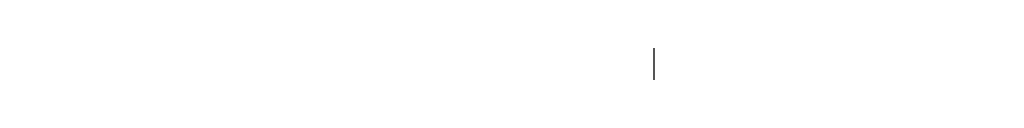
# Model space of a CAD drawing. Units: inches. Extents: x 2083 to 3317, y 1141 to 2115.
# Tile 63 of 256: x 2237.106 to 2238.294, y 1477.78 to 1477.8. Entities that reach past the tile are written whole.
import ezdxf

# ---------------------------------------------------------------- set-up
doc = ezdxf.new("R2010")
doc.units = ezdxf.units.IN
doc.layers.add('A-ANNO-DIMS', color=2, linetype='Continuous', lineweight=18)
doc.layers.add('A-WALL-PATT', color=251, linetype='Continuous', lineweight=13, true_color=0x636466)
doc.styles.get("Standard").update_dxf_attribs({"font": 'arial.ttf'})
doc.dimstyles.new('ISO-25', dxfattribs={"dimtxt": 12, "dimasz": 12, "dimexe": 1.25, "dimexo": 0.625, "dimtad": 1, "dimlunit": 3, "dimtxsty": 'Standard', "dimcen": 2.5, "dimadec": 0, "dimazin": 0, "dimtfac": 1, "dimtmove": 0, "dimatfit": 3, "dimfxl": 1, "dimarcsym": 0})

# ---------------------------------------------------------------- blocks, each defined once
blk = doc.blocks.new('*D30')
at = {"layer": 'A-ANNO-DIMS', "color": 0, "lineweight": -2, "transparency": 16777216}
for p, q in [((2240.0179, 1445.2738), (2240.0179, 1448.0455)), ((2254.3293, 1445.2738), (2254.3293, 1448.0455)), ((2228.0179, 1446.7955), (2216.0179, 1446.7955)), ((2240.0179, 1446.7955), (2254.3293, 1446.7955)), ((2266.3293, 1446.7955), (2413.7649, 1446.7955))]:
    blk.add_line(p, q, dxfattribs=at)
at = {"layer": 'A-ANNO-DIMS', "color": 0, "transparency": 16777216}
for points in [[(2228.0179, 1448.7955), (2228.0179, 1444.7955), (2240.0179, 1446.7955)], [(2266.3293, 1448.7955), (2266.3293, 1444.7955), (2254.3293, 1446.7955)]]:
    blk.add_solid(points, dxfattribs=at)
at = {"layer": 'Defpoints', "color": 0, "transparency": 16777216}
for p in [(2254.3293, 1446.7955), (2240.0179, 1444.6488), (2254.3293, 1444.6488)]:
    blk.add_point(p, dxfattribs=at)
at = {"layer": 'A-ANNO-DIMS', "color": 0, "transparency": 16777216, "insert": (2346.0471, 1453.6252), "char_height": 12, "attachment_point": 5}
blk.add_mtext('WC 1\'-2 1/2" TYP.', dxfattribs=at)
blk = doc.blocks.new('*D31')
at = {"layer": 'A-ANNO-DIMS', "color": 0, "lineweight": -2, "transparency": 16777216}
for p, q in [((2237.8711, 1456.6488), (2237.8711, 1541.9152)), ((2239.3929, 1444.6488), (2236.6211, 1444.6488)), ((2237.8711, 1431.5475), (2237.8711, 1444.6488)), ((2239.3929, 1431.5475), (2236.6211, 1431.5475)), ((2237.8711, 1419.5475), (2237.8711, 1407.5475))]:
    blk.add_line(p, q, dxfattribs=at)
at = {"layer": 'A-ANNO-DIMS', "color": 0, "transparency": 16777216}
for points in [[(2235.8711, 1456.6488), (2239.8711, 1456.6488), (2237.8711, 1444.6488)], [(2235.8711, 1419.5475), (2239.8711, 1419.5475), (2237.8711, 1431.5475)]]:
    blk.add_solid(points, dxfattribs=at)
at = {"layer": 'Defpoints', "color": 0, "transparency": 16777216}
for p in [(2237.8711, 1444.6488), (2240.0179, 1444.6488), (2240.0179, 1431.5475)]:
    blk.add_point(p, dxfattribs=at)
at = {"layer": 'A-ANNO-DIMS', "color": 0, "transparency": 16777216, "insert": (2231.2175, 1505.282), "char_height": 12, "attachment_point": 5, "rotation": 90}
blk.add_mtext('1\'-1" TYP.', dxfattribs=at)
blk = doc.blocks.new('*D45')
at = {"layer": 'A-ANNO-DIMS', "color": 0, "lineweight": -2, "transparency": 16777216}
for p, q in [((2235.9598, 1478.3864), (2235.9598, 1531.3614)), ((2418.9598, 1478.3864), (2418.9598, 1531.3614)), ((2247.9598, 1530.1114), (2406.9598, 1530.1114))]:
    blk.add_line(p, q, dxfattribs=at)
at = {"layer": 'A-ANNO-DIMS', "color": 0, "transparency": 16777216}
for points in [[(2247.9598, 1532.1114), (2247.9598, 1528.1114), (2235.9598, 1530.1114)], [(2406.9598, 1532.1114), (2406.9598, 1528.1114), (2418.9598, 1530.1114)]]:
    blk.add_solid(points, dxfattribs=at)
at = {"layer": 'Defpoints', "color": 0, "transparency": 16777216}
for p in [(2418.9598, 1530.1114), (2235.9598, 1477.7614), (2418.9598, 1477.7614)]:
    blk.add_point(p, dxfattribs=at)
at = {"layer": 'A-ANNO-DIMS', "color": 0, "transparency": 16777216, "insert": (2327.4598, 1536.8673), "char_height": 12, "attachment_point": 5}
blk.add_mtext('15\'-3"', dxfattribs=at)
blk = doc.blocks.new('*D62')
at = {"layer": 'A-ANNO-DIMS', "color": 0, "lineweight": -2, "transparency": 16777216}
for p, q in [((2235.9598, 1469.3864), (2235.9598, 1522.3614)), ((2379.9598, 1469.3864), (2379.9598, 1522.3614)), ((2247.9598, 1521.1114), (2367.9598, 1521.1114))]:
    blk.add_line(p, q, dxfattribs=at)
at = {"layer": 'A-ANNO-DIMS', "color": 0, "transparency": 16777216}
for points in [[(2247.9598, 1523.1114), (2247.9598, 1519.1114), (2235.9598, 1521.1114)], [(2367.9598, 1523.1114), (2367.9598, 1519.1114), (2379.9598, 1521.1114)]]:
    blk.add_solid(points, dxfattribs=at)
at = {"layer": 'Defpoints', "color": 0, "transparency": 16777216}
for p in [(2379.9598, 1521.1114), (2235.9598, 1468.7614), (2379.9598, 1468.7614)]:
    blk.add_point(p, dxfattribs=at)
at = {"layer": 'A-ANNO-DIMS', "color": 0, "transparency": 16777216, "insert": (2307.9598, 1527.8632), "char_height": 12, "attachment_point": 5}
blk.add_mtext('12\'-0"', dxfattribs=at)

msp = doc.modelspace()

# ---------------------------------------------------------------- hatches: boundary and pattern name
at = {"layer": 'A-WALL-PATT'}
h = msp.add_hatch(color=256, dxfattribs=at)
h.dxf.hatch_style = 1
h.paths.add_polyline_path([(3126.9598, 2020.7614), (2748.9598, 2020.7614), (2604.9598, 2020.7614), (2226.9598, 2020.7614), (2226.9598, 1702.7614), (2466.9598, 1702.7614), (2466.9598, 1582.7614), (2418.9598, 1582.7614), (2418.9598, 1477.7614), (2226.9598, 1477.7614), (2226.9598, 1263.2614), (2544.9598, 1263.2614), (2544.9598, 1411.7614), (2604.9598, 1411.7614), (2685.9598, 1411.7614), (2685.9598, 1420.7614), (2604.9598, 1420.7614), (2604.9598, 1573.7614), (2604.9598, 1702.7614), (2604.9598, 2011.7614), (2748.9598, 2011.7614), (2748.9598, 1702.7614), (2862.9598, 1702.7614), (2862.9598, 1621.7614), (2871.9598, 1621.7614), (2871.9598, 1702.7614), (2883.9598, 1702.7614), (2883.9598, 1706.9395, -0.026459), (2883.9598, 1711.7614), (2757.9598, 1711.7614), (2757.9598, 1807.7614), (2787.9598, 1807.7614), (2787.9598, 1812.2614), (2757.9598, 1812.2614), (2757.9598, 2011.7614), (2877.9598, 2011.7614), (2877.9598, 1812.2614), (2847.9598, 1812.2614), (2847.9598, 1807.7614), (2889.8357, 1807.7614), (2889.8357, 1812.2614), (2882.4598, 1812.2614), (2882.4598, 2011.7614), (3117.9598, 2011.7614), (3117.9598, 1812.2614), (2937.8357, 1812.2614), (2937.8357, 1807.7614), (2995.7098, 1807.7614), (2995.7098, 1796.1177), (3000.2098, 1796.1177), (3000.2098, 1807.7614), (3117.9598, 1807.7614), (3117.9598, 1711.7614), (3000.2098, 1711.7614), (3000.2098, 1760.1177), (2998.5727, 1760.1177, -0.020711), (2995.7098, 1760.1177), (2995.7098, 1711.7614), (2931.9598, 1711.7614), (2931.9598, 1702.7614), (3126.9598, 1702.7614)])
h.paths.add_polyline_path([(2471.4598, 2011.7614), (2471.4598, 1810.0114), (2462.7169, 1810.0114), (2462.7169, 1805.5114), (2505.9598, 1805.5114), (2505.9598, 1810.0114), (2475.9598, 1810.0114), (2475.9598, 2011.7614), (2595.9598, 2011.7614), (2595.9598, 1810.0114), (2565.9598, 1810.0114), (2565.9598, 1805.5114), (2595.9598, 1805.5114), (2595.9598, 1711.7614), (2235.9598, 1711.7614), (2235.9598, 1805.5114), (2353.7098, 1805.5114), (2353.7098, 1796.0542), (2358.2098, 1796.0542), (2358.2098, 1805.5114), (2414.7169, 1805.5114), (2414.7169, 1810.0114), (2235.9598, 1810.0114), (2235.9598, 2011.7614)], flags=16)
h.paths.add_polyline_path([(2270.2047, 1994.61), (2270.2047, 1970.61), (2246.2047, 1970.61), (2246.2047, 1994.61)], flags=0)
edge = h.paths.add_edge_path(flags=0)
edge.add_ellipse((2332.0274, 1899.7982), major_axis=(-3.043, 3.043), ratio=0.168252, start_angle=-161.3322, end_angle=-156.3071, ccw=False)
edge.add_ellipse((2333.082, 1898.7435), major_axis=(-1.0546, 1.0546), ratio=0.453532, start_angle=-123.371, end_angle=-94.1591)
edge = h.paths.add_edge_path(flags=0)
edge.add_ellipse((2332.0274, 1968.8763), major_axis=(3.043, 3.043), ratio=0.168252, start_angle=18.6678, end_angle=23.6929)
edge.add_spline(control_points=[(2332.9256, 1970.6911), (2332.2268, 1970.3361), (2330.8937, 1969.6589), (2328.4131, 1970.9321), (2327.2039, 1967.7487), (2324.7096, 1969.9556), (2322.5328, 1967.0124), (2320.0128, 1971.2958), (2317.6803, 1968.1578), (2316.0405, 1967.102), (2315.4269, 1966.8096)], knot_values=[0, 0, 0, 0, 2.267059, 4.324559, 6.685584, 8.878641, 11.121502, 14.300359, 17.755284, 19.732645, 19.732645, 19.732645, 19.732645], degree=3, periodic=0)
edge.add_ellipse((2332.0274, 1968.8763), major_axis=(3.043, 3.043), ratio=0.168252, start_angle=18.6678, end_angle=23.6929, ccw=False)
edge.add_ellipse((2333.082, 1969.9309), major_axis=(1.0546, 1.0546), ratio=0.453532, start_angle=56.629, end_angle=85.8409, ccw=False)
edge = h.paths.add_edge_path(flags=0)
edge.add_spline(control_points=[(2296.4283, 1967.9879), (2293.6278, 1965.3363), (2287.7036, 1959.7271), (2299.7439, 1949.9957), (2294.5326, 1935.6685), (2290.5732, 1920.6035), (2293.3941, 1909.9737), (2296.1854, 1904.9665)], knot_values=[0.099185, 0.099185, 0.099185, 0.099185, 0.345301, 0.619822, 0.982653, 1.386093, 1.810555, 1.810555, 1.810555, 1.810555], degree=3, periodic=0)
edge.add_spline(control_points=[(2296.1854, 1904.9665), (2297.3836, 1902.6193), (2298.001, 1901.9493), (2298.553, 1901.4682)], knot_values=[0.006246, 0.006246, 0.006246, 0.006246, 0.055476, 0.055476, 0.055476, 0.055476], degree=3, periodic=0)
edge.add_spline(control_points=[(2298.553, 1901.4682), (2297.2586, 1900.9232), (2295.2253, 1900.2321), (2293.0602, 1900.6142), (2292.1014, 1900.7884), (2292.0896, 1900.7906)], knot_values=[0.312835, 0.312835, 0.312835, 0.312835, 0.40178, 0.474987, 0.475903, 0.475903, 0.475903, 0.475903], degree=3, periodic=0)
edge.add_arc((2292.7936, 1904.6641), 3.937, 215.4209, 259.6982, ccw=False)
edge.add_spline(control_points=[(2289.5853, 1902.3823), (2289.4767, 1902.5351), (2289.3685, 1902.688), (2289.2609, 1902.8412)], knot_values=[0.102872, 0.102872, 0.102872, 0.102872, 0.116896, 0.116896, 0.116896, 0.116896], degree=3, periodic=0)
edge.add_spline(control_points=[(2289.2609, 1902.8412), (2288.6866, 1902.5502), (2287.64, 1902.0199), (2285.8813, 1901.874), (2283.853, 1901.5044), (2281.72, 1899.7105), (2278.467, 1899.4929), (2276.1571, 1901.8832), (2272.259, 1899.8041), (2267.7776, 1901.8432), (2262.2439, 1900.184), (2257.4149, 1901.7821), (2254.3184, 1900.7261), (2253.1783, 1900.3373)], knot_values=[0, 0, 0, 0, 1.907977, 3.477176, 5.261074, 7.972851, 11.680248, 13.717921, 16.939592, 22.789562, 27.502503, 33.595215, 37.145618, 37.145618, 37.145618, 37.145618], degree=3, periodic=0)
edge.add_line((2253.1783, 1900.3373), (2250.2442, 1902.8412))
edge.add_line((2250.2442, 1902.8412), (2250.2442, 1965.8333))
edge.add_line((2250.2442, 1965.8333), (2253.1783, 1968.3371))
edge.add_spline(control_points=[(2253.1783, 1968.3371), (2254.3184, 1967.9483), (2257.4149, 1966.8924), (2262.2439, 1968.4904), (2267.7776, 1966.8313), (2271.5267, 1968.5372), (2273.8759, 1967.8283), (2274.2067, 1967.7276)], knot_values=[0, 0, 0, 0, 0.09018, 0.244935, 0.364644, 0.513233, 0.537855, 0.537855, 0.537855, 0.537855], degree=3, periodic=0)
edge.add_arc((2274.3529, 1963.7933), 3.937, 72.0511, 92.1279, ccw=False)
edge.add_arc((2281.2969, 1985.23), 18.5963, 252.05113, 288.56572)
edge.add_arc((2292.3167, 1956.0289), 12.6461, 71.02679, 113.77822, ccw=False)
edge = h.paths.add_edge_path(flags=0)
edge.add_spline(control_points=[(2274.8994, 1951.8562), (2275.0662, 1951.6166), (2275.2327, 1951.3766), (2275.398, 1951.1359)], knot_values=[1.409916, 1.409916, 1.409916, 1.409916, 1.43159, 1.43159, 1.43159, 1.43159], degree=3, periodic=0)
edge.add_spline(control_points=[(2275.398, 1951.1359), (2275.7921, 1950.5619), (2276.1792, 1949.9838), (2276.5455, 1949.3971)], knot_values=[1.358238, 1.358238, 1.358238, 1.358238, 1.409916, 1.409916, 1.409916, 1.409916], degree=3, periodic=0)
edge.add_line((2276.5455, 1949.3971), (2277.4373, 1947.8622))
edge.add_spline(control_points=[(2277.4373, 1947.8622), (2276.3038, 1945.6731), (2274.6397, 1942.4269), (2274.6316, 1938.0939), (2272.7991, 1930.8515), (2274.3564, 1943.897), (2275.9477, 1947.9234), (2276.5455, 1949.3971)], knot_values=[0.005632, 0.005632, 0.005632, 0.005632, 0.186014, 0.266002, 0.357087, 0.59639, 0.739732, 0.739732, 0.739732, 0.739732], degree=3, periodic=0)
edge.add_spline(control_points=[(2276.5455, 1949.3971), (2276.1792, 1949.9838), (2275.7921, 1950.5619), (2275.398, 1951.1359)], knot_values=[1.358238, 1.358238, 1.358238, 1.358238, 1.409916, 1.409916, 1.409916, 1.409916], degree=3, periodic=0)
edge.add_spline(control_points=[(2275.398, 1951.1359), (2274.9425, 1950.0805), (2274.2078, 1948.0253), (2273.9346, 1944.8515), (2272.4685, 1937.6275), (2273.4662, 1945.6965), (2274.7006, 1951.0595), (2274.8994, 1951.8562)], knot_values=[0.104364, 0.104364, 0.104364, 0.104364, 0.189636, 0.269624, 0.36071, 0.600013, 0.644622, 0.644622, 0.644622, 0.644622], degree=3, periodic=0)
h.paths.add_polyline_path([(2269.1675, 1963.1276, -0.357527), (2268.1706, 1960.9764, -0.092561), (2268.1706, 1939.4363, -0.357527), (2269.1675, 1937.2851, -0.357527), (2267.0163, 1938.282, -0.164785), (2254.6856, 1938.282, -0.357527), (2252.5344, 1937.2851, -0.357527), (2253.5313, 1939.4363, -0.092561), (2253.5313, 1960.9764, -0.357527), (2252.5344, 1963.1276, -0.357527), (2254.6856, 1962.1307, -0.164785), (2267.0163, 1962.1307, -0.357527)], flags=0)
h.paths.add_polyline_path([(2248.8741, 1967.8018), (2248.8741, 1957.0277), (2249.4578, 1957.0277), (2249.4578, 1911.6468), (2248.8741, 1911.6468), (2248.8741, 1900.8727), (2246.5119, 1900.8727, 0.197327), (2244.1497, 1902.4569), (2244.1497, 1966.2176, 0.197327), (2246.5119, 1967.8018)], flags=0)
h.paths.add_polyline_path([(2269.1675, 1931.3893, -0.357527), (2268.1706, 1929.2381, -0.092561), (2268.1706, 1907.6981, -0.357527), (2269.1675, 1905.5469, -0.357527), (2267.0163, 1906.5438, -0.164785), (2254.6856, 1906.5438, -0.357527), (2252.5344, 1905.5469, -0.357527), (2253.5313, 1907.6981, -0.092561), (2253.5313, 1929.2381, -0.357527), (2252.5344, 1931.3893, -0.357527), (2254.6856, 1930.3925, -0.164785), (2267.0163, 1930.3925, -0.357527)], flags=0)
edge = h.paths.add_edge_path(flags=0)
edge.add_spline(control_points=[(2276.1969, 1906.7237), (2276.1681, 1909.0289), (2276.114, 1913.3719), (2270.5984, 1924.925), (2273.9052, 1919.0128), (2275.9217, 1916.2621), (2275.4746, 1912.4021), (2277.2579, 1910.3806), (2276.696, 1908.225), (2276.6462, 1906.813), (2276.6178, 1906.0084)], knot_values=[0, 0, 0, 0, 8.61026, 16.221274, 18.843057, 23.804898, 27.440828, 29.356102, 31.203478, 33.650687, 33.650687, 33.650687, 33.650687], degree=3, periodic=0)
edge.add_spline(control_points=[(2276.6178, 1906.0084), (2276.6233, 1905.6241), (2276.4977, 1904.6287), (2275.4418, 1903.8547), (2274.9373, 1903.0804), (2274.8591, 1902.8412)], knot_values=[0.156488, 0.156488, 0.156488, 0.156488, 0.184398, 0.231376, 0.250598, 0.250598, 0.250598, 0.250598], degree=3, periodic=0)
edge.add_line((2274.8591, 1902.8412), (2276.506, 1902.8412))
edge.add_spline(control_points=[(2276.506, 1902.8412), (2276.7883, 1903.0849), (2277.6651, 1904.1252), (2278.2495, 1904.3407), (2277.6539, 1908.5274), (2278.1557, 1906.2278), (2278.1005, 1905.2859), (2278.8467, 1904.069), (2277.8568, 1903.4149), (2277.8742, 1902.991), (2277.9036, 1902.8412)], knot_values=[0.059574, 0.059574, 0.059574, 0.059574, 0.080753, 0.103741, 0.16972, 0.176036, 0.207137, 0.240474, 0.262341, 0.27366, 0.27366, 0.27366, 0.27366], degree=3, periodic=0)
edge.add_line((2277.9036, 1902.8412), (2280.0298, 1902.8412))
edge.add_spline(control_points=[(2280.0298, 1902.8412), (2279.8882, 1903.0884), (2279.4993, 1903.9816), (2280.1523, 1905.9393), (2278.1036, 1909.6578), (2279.7624, 1907.1853), (2280.3279, 1904.8749), (2280.4851, 1903.4896), (2281.4633, 1903.2494), (2281.7583, 1902.9365), (2281.834, 1902.8412)], knot_values=[0.013856, 0.013856, 0.013856, 0.013856, 0.034874, 0.088867, 0.107879, 0.126738, 0.158714, 0.193757, 0.217487, 0.226722, 0.226722, 0.226722, 0.226722], degree=3, periodic=0)
edge.add_spline(control_points=[(2281.834, 1902.8412), (2281.7875, 1902.8267), (2281.647, 1902.783), (2281.3955, 1902.8595), (2281.0881, 1902.9852), (2280.7207, 1903.0609), (2280.3335, 1903.0257), (2280.1248, 1902.8989), (2280.0298, 1902.8412)], knot_values=[0, 0, 0, 0, 0.14413, 0.435517, 0.749276, 1.153046, 1.548371, 1.878348, 1.878348, 1.878348, 1.878348], degree=3, periodic=0)
edge.add_line((2280.0298, 1902.8412), (2277.9036, 1902.8412))
edge.add_spline(control_points=[(2277.9036, 1902.8412), (2277.8929, 1902.7959), (2277.8654, 1902.6796), (2277.6075, 1902.6875), (2277.2741, 1902.8007), (2276.8379, 1902.6198), (2276.5838, 1902.7893), (2276.506, 1902.8412)], knot_values=[0, 0, 0, 0, 0.127189, 0.326199, 0.628009, 1.24357, 1.515331, 1.515331, 1.515331, 1.515331], degree=3, periodic=0)
edge.add_line((2276.506, 1902.8412), (2274.8591, 1902.8412))
edge.add_spline(control_points=[(2274.8591, 1902.8412), (2274.8144, 1902.8986), (2274.7251, 1903.0134), (2274.4935, 1903.119), (2274.2443, 1902.9605), (2273.9371, 1903.1849), (2273.614, 1902.9831), (2273.4083, 1902.883), (2273.3223, 1902.8412)], knot_values=[0, 0, 0, 0, 0.21843, 0.436957, 0.687977, 0.990379, 1.398396, 1.69185, 1.69185, 1.69185, 1.69185], degree=3, periodic=0)
edge.add_spline(control_points=[(2273.3223, 1902.8412), (2273.6167, 1903.4457), (2274.274, 1904.5383), (2276.0272, 1904.5737), (2276.207, 1906.5836), (2276.1969, 1906.7237)], knot_values=[0.012227, 0.012227, 0.012227, 0.012227, 0.059472, 0.106218, 0.134458, 0.134458, 0.134458, 0.134458], degree=3, periodic=0)
h.paths.add_polyline_path([(2270.7761, 1897.7898), (2270.7761, 1873.7898), (2246.7761, 1873.7898), (2246.7761, 1897.7898)], flags=0)
h.paths.add_polyline_path([(2353.7098, 1760.0051), (2353.7098, 1760.0542), (2358.2098, 1760.0542, -0.033729)], flags=0)
h.paths.add_polyline_path([(2321.8191, 1737.5292), (2341.9953, 1737.5292, -0.414214), (2343.2033, 1736.3212), (2343.2033, 1721.0206, -0.414214), (2341.9953, 1719.8127), (2321.8191, 1719.8127, -0.414214), (2320.6112, 1721.0206), (2320.6112, 1736.3212, -0.414214)], flags=0)
h.paths.add_polyline_path([(2324.235, 1736.3212), (2339.5794, 1736.3212, -0.414214), (2341.9953, 1733.9053), (2341.9953, 1725.4497, -0.414214), (2339.5794, 1723.0338), (2333.6806, 1723.0338), (2333.8453, 1722.0455, -0.870646), (2335.4254, 1721.8259, -0.767327), (2333.9227, 1721.4232), (2331.291, 1721.4232, -0.767327), (2329.7883, 1721.8259, -0.870646), (2331.3684, 1722.0455), (2331.5331, 1723.0338), (2324.235, 1723.0338, -0.414214), (2321.8191, 1725.4497), (2321.8191, 1733.9053, -0.414214)], flags=0)
h.paths.add_polyline_path([(2570.4838, 1928.6154), (2589.6838, 1928.6154), (2590.1688, 1928.6154), (2590.1688, 1904.9934), (2570.4838, 1904.9934)], flags=0)
h.paths.add_polyline_path([(2574.4473, 1927.2638, -1), (2572.8288, 1927.2638, -1)], flags=0)
h.paths.add_polyline_path([(2573.0899, 1926.9409), (2573.925, 1927.776), (2574.1477, 1927.5533), (2573.3126, 1926.7182)], flags=0)
h.paths.add_polyline_path([(2578.7791, 1919.7296, -1), (2571.5917, 1919.7296, -1)], flags=0)
h.paths.add_polyline_path([(2578.3854, 1919.7296, -1), (2571.9854, 1919.7296, -1)], flags=0)
h.paths.add_polyline_path([(2331.5958, 1729.4762, -1), (2333.618, 1729.4762, -1)], flags=0)
h.paths.add_polyline_path([(2578.0342, 1927.2638, -1), (2576.4157, 1927.2638, -1)], flags=0)
h.paths.add_polyline_path([(2576.6889, 1927.5311), (2576.9116, 1927.7538), (2577.7467, 1926.9186), (2577.524, 1926.6959)], flags=0)
h.paths.add_polyline_path([(2578.1391, 1909.8595, -1), (2572.2317, 1909.8595, -1)], flags=0)
h.paths.add_polyline_path([(2577.7454, 1909.8595, -1), (2572.6254, 1909.8595, -1)], flags=0)
h.paths.add_polyline_path([(2583.7977, 1927.2638, -1), (2582.1792, 1927.2638, -1)], flags=0)
h.paths.add_polyline_path([(2582.7186, 1927.7538), (2583.5538, 1926.9186), (2583.3311, 1926.6959), (2582.4959, 1927.5311)], flags=0)
h.paths.add_polyline_path([(2582.4959, 1927.5311), (2582.7186, 1927.7538), (2583.5538, 1926.9186), (2583.3311, 1926.6959)], flags=0)
h.paths.add_polyline_path([(2587.7391, 1920.5296, -1), (2581.8317, 1920.5296, -1)], flags=0)
h.paths.add_polyline_path([(2587.3454, 1920.5296, -1), (2582.2254, 1920.5296, -1)], flags=0)
h.paths.add_polyline_path([(2587.3846, 1927.2638, -1), (2585.7661, 1927.2638, -1)], flags=0)
h.paths.add_polyline_path([(2586.082, 1926.9802), (2586.9172, 1927.8154), (2587.1399, 1927.5927), (2586.3047, 1926.7575)], flags=0)
h.paths.add_polyline_path([(2588.3791, 1910.6595, -1), (2581.1917, 1910.6595, -1)], flags=0)
h.paths.add_polyline_path([(2587.9854, 1910.6595, -1), (2581.5854, 1910.6595, -1)], flags=0)
h.paths.add_polyline_path([(2417.1677, 1729.4779), (2437.3439, 1729.4779, -0.414214), (2438.5519, 1728.2699), (2438.5519, 1712.9693, -0.414214), (2437.3439, 1711.7614), (2417.1677, 1711.7614, -0.414214), (2415.9598, 1712.9693), (2415.9598, 1728.2699, -0.414214)], flags=0)
h.paths.add_polyline_path([(2419.5836, 1728.2699), (2434.928, 1728.2699, -0.414214), (2437.3439, 1725.8541), (2437.3439, 1717.3984, -0.414214), (2434.928, 1714.9825), (2429.0292, 1714.9825), (2429.1939, 1713.9942, -0.870646), (2430.774, 1713.7746, -0.767327), (2429.2713, 1713.372), (2426.6396, 1713.372, -0.767327), (2425.1369, 1713.7746, -0.870646), (2426.717, 1713.9942), (2426.8817, 1714.9825), (2419.5836, 1714.9825, -0.414214), (2417.1677, 1717.3984), (2417.1677, 1725.8541, -0.414214)], flags=0)
h.paths.add_polyline_path([(2419.5836, 1728.2699), (2434.928, 1728.2699, -0.414214), (2437.3439, 1725.8541), (2437.3439, 1717.3984, -0.414214), (2434.928, 1714.9825), (2429.0292, 1714.9825), (2428.3581, 1719.009), (2427.5528, 1719.009), (2426.8817, 1714.9825), (2419.5836, 1714.9825, -0.414214), (2417.1677, 1717.3984), (2417.1677, 1725.8541, -0.414214)], flags=0)
h.paths.add_polyline_path([(2426.9444, 1721.4249, -1), (2428.9666, 1721.4249, -1)], flags=0)
h.paths.add_polyline_path([(2475.9598, 1702.7614), (2595.9598, 1702.7614), (2595.9598, 1582.7614), (2475.9598, 1582.7614)], flags=16)
h.paths.add_polyline_path([(2427.9598, 1573.7614), (2595.9598, 1573.7614), (2595.9598, 1468.7614), (2595.9598, 1420.7614), (2384.4598, 1420.7614), (2384.4598, 1468.7614), (2427.9598, 1468.7614)], flags=16)
h.paths.add_polyline_path([(2379.9598, 1468.7614), (2379.9598, 1420.7614), (2235.9598, 1420.7614), (2235.9598, 1468.7614)], flags=16)
h.paths.add_polyline_path([(2317.816, 1466.6958), (2337.9922, 1466.6958, -0.414214), (2339.2002, 1465.4878), (2339.2002, 1450.1872, -0.414214), (2337.9922, 1448.9792), (2317.816, 1448.9792, -0.414214), (2316.6081, 1450.1872), (2316.6081, 1465.4878, -0.414214)], flags=0)
h.paths.add_polyline_path([(2320.2319, 1465.4878), (2335.5763, 1465.4878, -0.414214), (2337.9922, 1463.0719), (2337.9922, 1454.6163, -0.414214), (2335.5763, 1452.2004), (2329.6775, 1452.2004), (2329.8422, 1451.212, -0.870646), (2331.4223, 1450.9925, -0.767327), (2329.9196, 1450.5898), (2327.2879, 1450.5898, -0.767327), (2325.7852, 1450.9925, -0.870646), (2327.3653, 1451.212), (2327.53, 1452.2004), (2320.2319, 1452.2004, -0.414214), (2317.816, 1454.6163), (2317.816, 1463.0719, -0.414214)], flags=0)
h.paths.add_polyline_path([(2320.2319, 1465.4878), (2335.5763, 1465.4878, -0.414214), (2337.9922, 1463.0719), (2337.9922, 1454.6163, -0.414214), (2335.5763, 1452.2004), (2329.6775, 1452.2004), (2329.0064, 1456.2269), (2328.2011, 1456.2269), (2327.53, 1452.2004), (2320.2319, 1452.2004, -0.414214), (2317.816, 1454.6163), (2317.816, 1463.0719, -0.414214)], flags=0)
h.paths.add_polyline_path([(2327.5926, 1458.6428, -1), (2329.6148, 1458.6428, -1)], flags=0)
h.paths.add_polyline_path([(2244.4117, 1433.3405), (2241.9209, 1433.3405, -0.414214), (2240.0179, 1435.2435), (2240.0179, 1440.9528, -0.414211), (2241.9209, 1442.8559), (2244.4117, 1442.8559, -1.976472)], flags=0)
h.paths.add_polyline_path([(2245.3569, 1434.3975, -0.414214), (2245.3569, 1441.7988, -2.144098)], flags=0)
h.paths.add_polyline_path([(2535.9598, 1416.2614), (2535.9598, 1272.2614), (2235.9598, 1272.2614), (2235.9598, 1416.2614)], flags=16)
h.paths.add_polyline_path([(2260.1196, 1384.2928), (2260.1196, 1362.0386), (2237.8654, 1362.0386), (2237.8654, 1384.2928)], flags=0)
edge = h.paths.add_edge_path(flags=0)
edge.add_line((2318.2518, 1362.0933), (2318.1458, 1362.001))
edge.add_ellipse((2317.4451, 1360.431), major_axis=(2.8216, 2.8216), ratio=0.168252, start_angle=18.6678, end_angle=20.9481, ccw=False)
edge.add_ellipse((2318.423, 1361.409), major_axis=(0.9779, 0.9779), ratio=0.453532, start_angle=56.629, end_angle=70.2262, ccw=False)
edge = h.paths.add_edge_path(flags=0)
edge.add_line((2319.1074, 1295.5711), (2319.015, 1295.6771))
edge.add_ellipse((2317.4451, 1296.3778), major_axis=(-2.8216, 2.8216), ratio=0.168252, start_angle=-161.3322, end_angle=-159.0519, ccw=False)
edge.add_ellipse((2318.423, 1295.3999), major_axis=(-0.9779, 0.9779), ratio=0.453532, start_angle=-123.371, end_angle=-109.7738)
edge = h.paths.add_edge_path(flags=0)
edge.add_spline(control_points=[(2284.2103, 1301.1702), (2284.5807, 1300.4447), (2284.8912, 1299.892), (2285.1596, 1299.461)], knot_values=[0.039066, 0.039066, 0.039066, 0.039066, 0.055476, 0.055476, 0.055476, 0.055476], degree=3, periodic=0)
edge.add_line((2285.1596, 1299.461), (2284.2103, 1301.1702))
edge = h.paths.add_edge_path(flags=0)
edge.add_line((2280.4125, 1297.298), (2283.37, 1297.0361))
edge.add_line((2283.37, 1297.0361), (2286.4057, 1297.9263))
edge.add_spline(control_points=[(2286.4057, 1297.9263), (2285.3055, 1297.4631), (2284.3448, 1297.1292), (2283.37, 1297.0361)], knot_values=[0.394369, 0.394369, 0.394369, 0.394369, 0.475903, 0.475903, 0.475903, 0.475903], degree=3, periodic=0)
edge.add_spline(control_points=[(2283.37, 1297.0361), (2283.2814, 1297.0277), (2282.3163, 1296.9573), (2281.3125, 1297.1345), (2280.4234, 1297.296), (2280.4125, 1297.298)], knot_values=[0.312835, 0.312835, 0.312835, 0.312835, 0.320246, 0.393453, 0.394369, 0.394369, 0.394369, 0.394369], degree=3, periodic=0)
edge = h.paths.add_edge_path(flags=0)
edge.add_line((2284.4356, 1359.6073), (2280.4463, 1355.328))
edge.add_line((2280.4463, 1355.328), (2279.58, 1351.0178))
edge.add_line((2279.58, 1351.0178), (2282.413, 1346.5804))
edge.add_spline(control_points=[(2282.413, 1346.5804), (2283.1533, 1345.5892), (2284.2529, 1344.0289), (2284.801, 1342.3872), (2284.9352, 1341.8055)], knot_values=[1.240098, 1.240098, 1.240098, 1.240098, 1.332892, 1.382712, 1.382712, 1.382712, 1.382712], degree=3, periodic=0)
edge.add_spline(control_points=[(2284.9352, 1341.8055), (2285.3191, 1340.1406), (2285.233, 1338.4092), (2284.9099, 1336.6541)], knot_values=[1.097484, 1.097484, 1.097484, 1.097484, 1.240098, 1.240098, 1.240098, 1.240098], degree=3, periodic=0)
edge.add_spline(control_points=[(2284.9099, 1336.6541), (2284.5868, 1334.899), (2284.0267, 1333.1203), (2283.4626, 1331.3606)], knot_values=[0.95487, 0.95487, 0.95487, 0.95487, 1.097484, 1.097484, 1.097484, 1.097484], degree=3, periodic=0)
edge.add_line((2283.4626, 1331.3606), (2281.8904, 1326.1534))
edge.add_line((2281.8904, 1326.1534), (2280.7563, 1321.0561))
edge.add_line((2280.7563, 1321.0561), (2280.2992, 1316.002))
edge.add_line((2280.2992, 1316.002), (2280.7159, 1310.9501))
edge.add_line((2280.7159, 1310.9501), (2282.0281, 1305.9721))
edge.add_line((2282.0281, 1305.9721), (2284.2103, 1301.1702))
edge.add_spline(control_points=[(2284.2103, 1301.1702), (2283.3407, 1302.7302), (2282.6119, 1304.3365), (2282.0281, 1305.9721)], knot_values=[0.099185, 0.099185, 0.099185, 0.099185, 0.241799, 0.241799, 0.241799, 0.241799], degree=3, periodic=0)
edge.add_spline(control_points=[(2282.0281, 1305.9721), (2281.4443, 1307.6078), (2281.0055, 1309.2728), (2280.7159, 1310.9501)], knot_values=[0.241799, 0.241799, 0.241799, 0.241799, 0.384413, 0.384413, 0.384413, 0.384413], degree=3, periodic=0)
edge.add_spline(control_points=[(2280.7159, 1310.9501), (2280.4332, 1312.5876), (2280.2894, 1314.277), (2280.2989, 1315.962), (2280.2992, 1316.002)], knot_values=[0.384413, 0.384413, 0.384413, 0.384413, 0.523647, 0.527028, 0.527028, 0.527028, 0.527028], degree=3, periodic=0)
edge.add_spline(control_points=[(2280.2992, 1316.002), (2280.3123, 1317.687), (2280.4779, 1319.3679), (2280.7563, 1321.0561)], knot_values=[0.527028, 0.527028, 0.527028, 0.527028, 0.669642, 0.669642, 0.669642, 0.669642], degree=3, periodic=0)
edge.add_spline(control_points=[(2280.7563, 1321.0561), (2281.0346, 1322.7443), (2281.4259, 1324.4396), (2281.8904, 1326.1534)], knot_values=[0.669642, 0.669642, 0.669642, 0.669642, 0.812256, 0.812256, 0.812256, 0.812256], degree=3, periodic=0)
edge.add_spline(control_points=[(2281.8904, 1326.1534), (2282.2644, 1327.5333), (2282.7879, 1329.2618), (2283.3528, 1331.0178), (2283.4626, 1331.3606)], knot_values=[0.812256, 0.812256, 0.812256, 0.812256, 0.927087, 0.95487, 0.95487, 0.95487, 0.95487], degree=3, periodic=0)
edge.add_line((2283.4626, 1331.3606), (2284.9099, 1336.6541))
edge.add_line((2284.9099, 1336.6541), (2284.9352, 1341.8055))
edge.add_line((2284.9352, 1341.8055), (2282.413, 1346.5804))
edge.add_spline(control_points=[(2282.413, 1346.5804), (2281.2751, 1348.1038), (2280.0784, 1349.5703), (2279.58, 1351.0178)], knot_values=[1.382712, 1.382712, 1.382712, 1.382712, 1.525326, 1.525326, 1.525326, 1.525326], degree=3, periodic=0)
edge.add_spline(control_points=[(2279.58, 1351.0178), (2279.4433, 1351.4147), (2279.1363, 1352.8569), (2279.7352, 1354.2904), (2280.4463, 1355.328)], knot_values=[1.525326, 1.525326, 1.525326, 1.525326, 1.564439, 1.667941, 1.667941, 1.667941, 1.667941], degree=3, periodic=0)
edge.add_spline(control_points=[(2280.4463, 1355.328), (2281.4261, 1356.7578), (2282.9308, 1358.1826), (2284.4356, 1359.6073)], knot_values=[1.667941, 1.667941, 1.667941, 1.667941, 1.810555, 1.810555, 1.810555, 1.810555], degree=3, periodic=0)
edge.add_arc((2280.6231, 1348.5182), 11.7262, 71.02679, 113.77822)
edge.add_arc((2270.4049, 1375.5952), 17.2436, 252.05113, 288.56572, ccw=False)
edge.add_arc((2263.966, 1355.7178), 3.6506, 72.0511, 92.1279)
edge.add_arc((2263.966, 1355.7178), 3.6506, 92.1279, 177.9851)
edge.add_spline(control_points=[(2260.3176, 1355.8462), (2260.2604, 1354.2207), (2260.5513, 1350.1865), (2262.9993, 1346.7663), (2264.4727, 1344.649)], knot_values=[1.43159, 1.43159, 1.43159, 1.43159, 1.564144, 1.770695, 1.770695, 1.770695, 1.770695], degree=3, periodic=0)
edge.add_line((2264.4727, 1344.649), (2264.9356, 1343.9825))
edge.add_spline(control_points=[(2263.801, 1340.2481), (2263.8432, 1340.5141), (2264.0672, 1341.7565), (2264.5127, 1343.0025), (2264.935, 1343.9811)], knot_values=[0.53657, 0.53657, 0.53657, 0.53657, 0.559349, 0.644622, 0.644622, 0.644622, 0.644622], degree=3, periodic=0)
edge.add_spline(control_points=[(2264.935, 1343.9811), (2265.1178, 1343.715), (2265.2989, 1343.4479), (2265.4768, 1343.1794)], knot_values=[1.384077, 1.384077, 1.384077, 1.384077, 1.409916, 1.409916, 1.409916, 1.409916], degree=3, periodic=0)
edge.add_spline(control_points=[(2265.4768, 1343.1794), (2265.6546, 1342.9108), (2265.8293, 1342.6408), (2265.9991, 1342.3688)], knot_values=[1.358238, 1.358238, 1.358238, 1.358238, 1.384077, 1.384077, 1.384077, 1.384077], degree=3, periodic=0)
edge.add_line((2265.9991, 1342.3688), (2266.826, 1340.9455))
edge.add_spline(control_points=[(2266.826, 1340.9455), (2268.8944, 1337.0897), (2271.3982, 1325.843), (2270.5162, 1310.5686), (2275.9194, 1301.8606), (2277.7895, 1299.1994)], knot_values=[0.116896, 0.116896, 0.116896, 0.116896, 0.472987, 1.050969, 1.313793, 1.313793, 1.313793, 1.313793], degree=3, periodic=0)
edge.add_spline(control_points=[(2277.7895, 1299.1994), (2277.8394, 1299.1285), (2277.8894, 1299.0575), (2277.9396, 1298.9866)], knot_values=[0.109884, 0.109884, 0.109884, 0.109884, 0.116896, 0.116896, 0.116896, 0.116896], degree=3, periodic=0)
edge.add_line((2277.9396, 1298.9866), (2277.7888, 1299.1991))
edge.add_spline(control_points=[(2277.7888, 1299.1991), (2277.2566, 1298.9294), (2276.2864, 1298.4379), (2275.0394, 1298.3344), (2274.3833, 1298.2389), (2274.2153, 1298.2093)], knot_values=[33.12187, 33.12187, 33.12187, 33.12187, 35.029056, 36.598255, 37.144827, 37.144827, 37.144827, 37.144827], degree=3, periodic=0)
edge.add_line((2274.2153, 1298.2093), (2273.0731, 1297.893))
edge.add_spline(control_points=[(2273.0731, 1297.893), (2272.3229, 1297.5798), (2271.0392, 1296.5105), (2269.2484, 1296.2261), (2268.4231, 1296.3747)], knot_values=[26.532584, 26.532584, 26.532584, 26.532584, 29.198919, 31.839101, 31.839101, 31.839101, 31.839101], degree=3, periodic=0)
edge.add_line((2268.4231, 1296.3747), (2263.8785, 1297.4575))
edge.add_spline(control_points=[(2263.8785, 1297.4575), (2263.5561, 1297.3594), (2261.8603, 1296.8387), (2260.2388, 1297.2824), (2258.9335, 1297.5165)], knot_values=[15.919551, 15.919551, 15.919551, 15.919551, 16.939592, 21.226067, 21.226067, 21.226067, 21.226067], degree=3, periodic=0)
edge.add_line((2258.9335, 1297.5165), (2254.0552, 1297.329))
edge.add_spline(control_points=[(2254.0552, 1297.329), (2253.7555, 1297.2958), (2252.1137, 1297.1652), (2250.4619, 1297.5442), (2249.1297, 1297.6679)], knot_values=[5.306517, 5.306517, 5.306517, 5.306517, 6.276435, 10.613034, 10.613034, 10.613034, 10.613034], degree=3, periodic=0)
edge.add_line((2249.1297, 1297.6679), (2244.3316, 1296.8778))
edge.add_line((2244.3316, 1296.8778), (2241.611, 1299.1994))
edge.add_line((2241.611, 1299.1994), (2241.611, 1357.6094))
edge.add_line((2241.611, 1357.6094), (2244.3316, 1359.9311))
edge.add_line((2244.3316, 1359.9311), (2252.7288, 1359.5427))
edge.add_spline(control_points=[(2252.7288, 1359.5427), (2252.8709, 1359.5464), (2253.3057, 1359.5482), (2253.7398, 1359.5143), (2254.0317, 1359.4824)], knot_values=[0.233291, 0.233291, 0.233291, 0.233291, 0.244935, 0.268927, 0.268927, 0.268927, 0.268927], degree=3, periodic=0)
edge.add_line((2254.0317, 1359.4824), (2259.5872, 1359.4164))
edge.add_spline(control_points=[(2259.5872, 1359.4164), (2260.6771, 1359.6285), (2262.0732, 1359.897), (2263.5237, 1359.4593), (2263.8304, 1359.366)], knot_values=[0.422516, 0.422516, 0.422516, 0.422516, 0.513233, 0.537855, 0.537855, 0.537855, 0.537855], degree=3, periodic=0)
edge.add_arc((2263.966, 1355.7178), 3.6506, 72.0511, 92.1279, ccw=False)
edge.add_arc((2270.4049, 1375.5952), 17.2436, 252.05113, 288.56572)
edge.add_arc((2280.6231, 1348.5182), 11.7262, 71.02679, 113.77822, ccw=False)
h.paths.add_polyline_path([(2240.3405, 1359.4347), (2240.3405, 1349.4444), (2240.8818, 1349.4444), (2240.8818, 1307.3645), (2240.3405, 1307.3645), (2240.3405, 1297.3741), (2238.1502, 1297.3741, 0.197327), (2235.9598, 1298.8431), (2235.9598, 1357.9657, 0.197327), (2238.1502, 1359.4347)], flags=0)
h.paths.add_polyline_path([(2259.1578, 1355.1005, -0.357527), (2258.2334, 1353.1058, -0.092561), (2258.2334, 1333.1326, -0.357527), (2259.1578, 1331.1379, -0.357527), (2257.1631, 1332.0622, -0.164785), (2245.7293, 1332.0622, -0.357527), (2243.7346, 1331.1379, -0.357527), (2244.6589, 1333.1326, -0.092561), (2244.6589, 1353.1058, -0.357527), (2243.7346, 1355.1005, -0.357527), (2245.7293, 1354.1761, -0.164785), (2257.1631, 1354.1761, -0.357527)], flags=0)
edge = h.paths.add_edge_path(flags=0)
edge.add_line((2265.9991, 1342.3688), (2266.826, 1340.9455))
edge.add_line((2266.826, 1340.9455), (2265.3076, 1337.8141))
edge.add_line((2265.3076, 1337.8141), (2264.3582, 1334.6529))
edge.add_line((2264.3582, 1334.6529), (2264.262, 1333.7997))
edge.add_spline(control_points=[(2264.262, 1333.7997), (2264.2084, 1333.1871), (2264.1621, 1332.3655), (2264.0071, 1331.4139), (2263.969, 1331.2018)], knot_values=[0.464444, 0.464444, 0.464444, 0.464444, 0.516691, 0.531608, 0.531608, 0.531608, 0.531608], degree=3, periodic=0)
edge.add_spline(control_points=[(2263.969, 1331.2018), (2263.7745, 1330.1189), (2263.4244, 1328.7908), (2263.2574, 1328.5307), (2263.234, 1328.5146)], knot_values=[0.372682, 0.372682, 0.372682, 0.372682, 0.44885, 0.464444, 0.464444, 0.464444, 0.464444], degree=3, periodic=0)
edge.add_spline(control_points=[(2263.234, 1328.5146), (2263.0964, 1328.4202), (2263.1312, 1329.3015), (2263.275, 1330.6157)], knot_values=[0.280919, 0.280919, 0.280919, 0.280919, 0.372682, 0.372682, 0.372682, 0.372682], degree=3, periodic=0)
edge.add_spline(control_points=[(2263.275, 1330.6157), (2263.4187, 1331.93), (2263.6715, 1333.6773), (2263.9699, 1335.315)], knot_values=[0.189157, 0.189157, 0.189157, 0.189157, 0.280919, 0.280919, 0.280919, 0.280919], degree=3, periodic=0)
edge.add_spline(control_points=[(2263.9699, 1335.315), (2264.1005, 1336.0322), (2264.4188, 1337.6219), (2264.7548, 1338.8644), (2264.9474, 1339.4911)], knot_values=[0.097394, 0.097394, 0.097394, 0.097394, 0.137578, 0.189157, 0.189157, 0.189157, 0.189157], degree=3, periodic=0)
edge.add_spline(control_points=[(2264.9474, 1339.4911), (2265.29, 1340.6061), (2265.6442, 1341.494), (2265.9991, 1342.3688)], knot_values=[0.005632, 0.005632, 0.005632, 0.005632, 0.097394, 0.097394, 0.097394, 0.097394], degree=3, periodic=0)
h.paths.add_polyline_path([(2259.1578, 1325.671, -0.357527), (2258.2334, 1323.6763, -0.092561), (2258.2334, 1303.7031, -0.357527), (2259.1578, 1301.7084, -0.357527), (2257.1631, 1302.6327, -0.164785), (2245.7293, 1302.6327, -0.357527), (2243.7346, 1301.7084, -0.357527), (2244.6589, 1303.7031, -0.092561), (2244.6589, 1323.6763, -0.357527), (2243.7346, 1325.671, -0.357527), (2245.7293, 1324.7466, -0.164785), (2257.1631, 1324.7466, -0.357527)], flags=0)
edge = h.paths.add_edge_path(flags=0)
edge.add_spline(control_points=[(2261.7089, 1317.3114), (2261.6795, 1317.4176), (2261.7619, 1317.3885), (2262.4907, 1316.0899), (2262.9622, 1315.3009)], knot_values=[14.955861, 14.955861, 14.955861, 14.955861, 16.221274, 18.694826, 18.694826, 18.694826, 18.694826], degree=3, periodic=0)
edge.add_spline(control_points=[(2262.9622, 1315.3009), (2262.9904, 1315.2536), (2263.7021, 1314.0674), (2264.349, 1313.1272), (2264.7301, 1312.1642)], knot_values=[18.694826, 18.694826, 18.694826, 18.694826, 18.843057, 22.433791, 22.433791, 22.433791, 22.433791], degree=3, periodic=0)
edge.add_spline(control_points=[(2264.7301, 1312.1642), (2264.8756, 1311.7964), (2265.1769, 1310.7698), (2265.1431, 1309.5593), (2265.2477, 1308.8242)], knot_values=[22.433791, 22.433791, 22.433791, 22.433791, 23.804898, 26.172756, 26.172756, 26.172756, 26.172756], degree=3, periodic=0)
edge.add_line((2265.2477, 1308.8242), (2265.8508, 1307.1719))
edge.add_spline(control_points=[(2265.8508, 1307.1719), (2266.065, 1306.8217), (2266.3844, 1306.3322), (2266.4244, 1305.7805), (2266.4204, 1305.6112)], knot_values=[28.062562, 28.062562, 28.062562, 28.062562, 29.356102, 29.911721, 29.911721, 29.911721, 29.911721], degree=3, periodic=0)
edge.add_spline(control_points=[(2266.4204, 1305.6112), (2266.4161, 1305.4326), (2266.394, 1305.25), (2266.3648, 1305.0659)], knot_values=[29.911721, 29.911721, 29.911721, 29.911721, 30.497837, 30.497837, 30.497837, 30.497837], degree=3, periodic=0)
edge.add_line((2266.3648, 1305.0659), (2266.0662, 1302.1363))
edge.add_spline(control_points=[(2266.0662, 1302.1363), (2266.0712, 1301.78), (2265.9981, 1301.2), (2265.6633, 1300.759), (2265.5089, 1300.5859)], knot_values=[0.156488, 0.156488, 0.156488, 0.156488, 0.184398, 0.203543, 0.203543, 0.203543, 0.203543], degree=3, periodic=0)
edge.add_line((2265.5089, 1300.5859), (2264.4353, 1299.1994))
edge.add_line((2264.4353, 1299.1994), (2265.9624, 1299.1994))
edge.add_line((2265.9624, 1299.1994), (2267.336, 1301.1753))
edge.add_line((2267.336, 1301.1753), (2267.3117, 1301.9862))
edge.add_spline(control_points=[(2267.3117, 1301.9862), (2267.2611, 1302.8624), (2267.1602, 1303.7371), (2267.2715, 1303.3259)], knot_values=[0.126229, 0.126229, 0.126229, 0.126229, 0.166617, 0.166617, 0.166617, 0.166617], degree=3, periodic=0)
edge.add_spline(control_points=[(2267.2715, 1303.3259), (2267.28, 1303.2943), (2267.3098, 1303.1754), (2267.3735, 1302.8836), (2267.4061, 1302.6828), (2267.4179, 1302.601)], knot_values=[0.166617, 0.166617, 0.166617, 0.166617, 0.16972, 0.176036, 0.180765, 0.180765, 0.180765, 0.180765], degree=3, periodic=0)
edge.add_spline(control_points=[(2267.7439, 1300.9875), (2267.6876, 1301.1509), (2267.4805, 1301.6567), (2267.4838, 1302.1448), (2267.4179, 1302.601)], knot_values=[0.180765, 0.180765, 0.180765, 0.180765, 0.193767, 0.220139, 0.220139, 0.220139, 0.220139], degree=3, periodic=0)
edge.add_line((2267.4179, 1302.601), (2267.7439, 1300.9875))
edge.add_spline(control_points=[(2267.7439, 1300.9875), (2267.832, 1300.7319), (2267.932, 1300.3099), (2267.5548, 1299.9745), (2267.4294, 1299.8292)], knot_values=[0.220139, 0.220139, 0.220139, 0.220139, 0.240474, 0.25489, 0.25489, 0.25489, 0.25489], degree=3, periodic=0)
edge.add_line((2267.4294, 1299.8292), (2267.2584, 1299.1994))
edge.add_line((2267.2584, 1299.1994), (2269.23, 1299.1994))
edge.add_spline(control_points=[(2269.23, 1299.1994), (2269.0987, 1299.4287), (2268.8428, 1300.0163), (2269.0116, 1300.9159), (2268.9468, 1301.6607)], knot_values=[0.013856, 0.013856, 0.013856, 0.013856, 0.034874, 0.067073, 0.067073, 0.067073, 0.067073], degree=3, periodic=0)
edge.add_line((2268.9468, 1301.6607), (2268.4316, 1303.6031))
edge.add_spline(control_points=[(2268.4316, 1303.6031), (2268.1756, 1304.1924), (2267.5962, 1305.2513), (2268.0407, 1304.6232), (2268.2514, 1304.2824)], knot_values=[0.090155, 0.090155, 0.090155, 0.090155, 0.107879, 0.120289, 0.120289, 0.120289, 0.120289], degree=3, periodic=0)
edge.add_spline(control_points=[(2268.2514, 1304.2824), (2268.3609, 1304.1053), (2269.0578, 1302.918), (2269.3827, 1301.5904), (2269.5214, 1300.7759), (2269.5752, 1300.5558)], knot_values=[0.120289, 0.120289, 0.120289, 0.120289, 0.126738, 0.158714, 0.173506, 0.173506, 0.173506, 0.173506], degree=3, periodic=0)
edge.add_line((2269.5752, 1300.5558), (2270.6858, 1299.4213))
edge.add_spline(control_points=[(2270.6858, 1299.4213), (2270.7672, 1299.3573), (2270.8379, 1299.2814), (2270.9029, 1299.1994)], knot_values=[0.21816, 0.21816, 0.21816, 0.21816, 0.226722, 0.226722, 0.226722, 0.226722], degree=3, periodic=0)
edge.add_line((2270.9372, 1299.1929), (2270.9029, 1299.1994))
edge.add_spline(control_points=[(2270.9029, 1299.1994), (2270.8598, 1299.186), (2270.7295, 1299.1455), (2270.4963, 1299.2164), (2270.2717, 1299.3083), (2270.121, 1299.348), (2270.0633, 1299.3596)], knot_values=[0.939174, 0.939174, 0.939174, 0.939174, 1.083304, 1.374691, 1.68845, 1.878348, 1.878348, 1.878348, 1.878348], degree=3, periodic=0)
edge.add_line((2270.0633, 1299.3596), (2269.23, 1299.1994))
edge.add_line((2269.23, 1299.1994), (2267.2584, 1299.1994))
edge.add_spline(control_points=[(2267.2584, 1299.1994), (2267.2484, 1299.1574), (2267.223, 1299.0497), (2266.9838, 1299.0569), (2266.8092, 1299.1162), (2266.6769, 1299.1091), (2266.6365, 1299.1048)], knot_values=[0.757665, 0.757665, 0.757665, 0.757665, 0.884854, 1.083864, 1.385675, 1.515331, 1.515331, 1.515331, 1.515331], degree=3, periodic=0)
edge.add_spline(control_points=[(2266.6365, 1299.1048), (2266.4852, 1299.0888), (2266.2358, 1299.0171), (2266.0346, 1299.1513), (2265.9624, 1299.1994)], knot_values=[0, 0, 0, 0, 0.485905, 0.757665, 0.757665, 0.757665, 0.757665], degree=3, periodic=0)
edge.add_line((2265.9624, 1299.1994), (2264.4353, 1299.1994))
edge.add_line((2264.4353, 1299.1994), (2263.8584, 1299.3671))
edge.add_spline(control_points=[(2263.8584, 1299.3671), (2263.8189, 1299.3709), (2263.7795, 1299.3857), (2263.7401, 1299.4015)], knot_values=[0.845925, 0.845925, 0.845925, 0.845925, 0.978627, 0.978627, 0.978627, 0.978627], degree=3, periodic=0)
edge.add_line((2263.7218, 1299.3964), (2263.0103, 1299.1994))
edge.add_spline(control_points=[(2263.0103, 1299.1994), (2263.2458, 1299.6829), (2263.506, 1300.1281), (2263.8735, 1300.408)], knot_values=[0.012227, 0.012227, 0.012227, 0.012227, 0.052971, 0.052971, 0.052971, 0.052971], degree=3, periodic=0)
edge.add_spline(control_points=[(2263.8735, 1300.408), (2263.9321, 1300.4527), (2264.0842, 1300.553), (2264.2552, 1300.6242), (2264.3597, 1300.6647)], knot_values=[0.052971, 0.052971, 0.052971, 0.052971, 0.059472, 0.069086, 0.069086, 0.069086, 0.069086], degree=3, periodic=0)
edge.add_line((2264.3597, 1300.6647), (2265.1419, 1301.0778))
edge.add_line((2265.1419, 1301.0778), (2265.6758, 1302.7996))
edge.add_line((2265.6758, 1302.7996), (2265.5407, 1305.7041))
edge.add_line((2265.5407, 1305.7041), (2264.8031, 1309.3277))
edge.add_line((2264.8031, 1309.3277), (2263.0405, 1314.0918))
edge.add_spline(control_points=[(2263.0405, 1314.0918), (2262.3836, 1315.6714), (2261.796, 1316.9977), (2261.7089, 1317.3114)], knot_values=[11.216896, 11.216896, 11.216896, 11.216896, 14.955861, 14.955861, 14.955861, 14.955861], degree=3, periodic=0)
h.paths.add_polyline_path([(2871.9598, 1416.2614), (2895.91, 1416.2614), (2895.91, 1420.7614), (2871.9598, 1420.7614), (2871.9598, 1501.7614), (2862.9598, 1501.7614), (2862.9598, 1420.7614), (2805.9598, 1420.7614), (2805.9598, 1411.7614), (2862.9598, 1411.7614), (2862.9598, 1263.2614), (3126.9598, 1263.2614), (3126.9598, 1411.7614), (3126.9598, 1486.7614), (2943.9598, 1486.7614), (2943.9598, 1477.7614), (2967.8603, 1477.7614), (2967.8603, 1420.7614), (2943.91, 1420.7614), (2943.91, 1416.2614), (3117.9598, 1416.2614), (3117.9598, 1420.7614), (2972.3603, 1420.7614), (2972.3603, 1477.7614), (3117.9598, 1477.7614), (3117.9598, 1420.7614), (3117.9598, 1272.2614), (2871.9598, 1272.2614)], flags=0)
h.paths.add_polyline_path([(2457.1256, 1485.9425), (2527.6027, 1485.9425), (2527.6027, 1537.6357), (2457.1256, 1537.6357)], flags=8)
h.paths.add_polyline_path([(2481.0051, 1609.9818), (2590.7658, 1609.9818), (2590.7658, 1682.0034), (2481.0051, 1682.0034)], flags=8)
h.paths.add_polyline_path([(2483.085, 1729.1268), (2553.562, 1729.1268), (2553.562, 1780.82), (2483.085, 1780.82)], flags=8)

# ---------------------------------------------------------------- dimensions: what is measured, and where the dimension line sits
at = {"layer": 'A-ANNO-DIMS'}
for base, p1, p2, picture, middle in [((2418.9598, 1530.1114), (2235.9598, 1477.7614), (2418.9598, 1477.7614), '*D45', (2327.4598, 1536.8673)), ((2379.9598, 1521.1114), (2235.9598, 1468.7614), (2379.9598, 1468.7614), '*D62', (2307.9598, 1527.8632))]:
    dim = msp.add_linear_dim(base=base, p1=p1, p2=p2, dimstyle='ISO-25', override={"dimdec": 1, "dimlfac": 1, "dimrnd": 0, "dimzin": 1, "dimdsep": 46, "dimlunit": 4, "dimfrac": 2}, dxfattribs=at)
    dim.commit()
    dim.dimension.update_dxf_attribs({"geometry": picture, "text_midpoint": middle})
dim = msp.add_linear_dim(base=(2237.8711, 1444.6488), p1=(2240.0179, 1431.5475), p2=(2240.0179, 1444.6488), angle=90, text='<> TYP.', dimstyle='ISO-25', override={"dimdec": 1, "dimlfac": 1, "dimrnd": 0, "dimzin": 1, "dimdsep": 46, "dimlunit": 4, "dimfrac": 2}, dxfattribs=at)
dim.commit()
dim.dimension.update_dxf_attribs({"geometry": '*D31', "text_midpoint": (2231.2175, 1505.282)})
dim = msp.add_linear_dim(base=(2254.3293, 1446.7955), p1=(2240.0179, 1444.6488), p2=(2254.3293, 1444.6488), text='WC <> TYP.', dimstyle='ISO-25', override={"dimdec": 1, "dimlfac": 1, "dimrnd": 0, "dimzin": 1, "dimdsep": 46, "dimlunit": 4, "dimfrac": 2}, dxfattribs=at)
dim.commit()
dim.dimension.update_dxf_attribs({"geometry": '*D30', "text_midpoint": (2346.0471, 1453.6252)})

doc.saveas('drawing.dxf')
